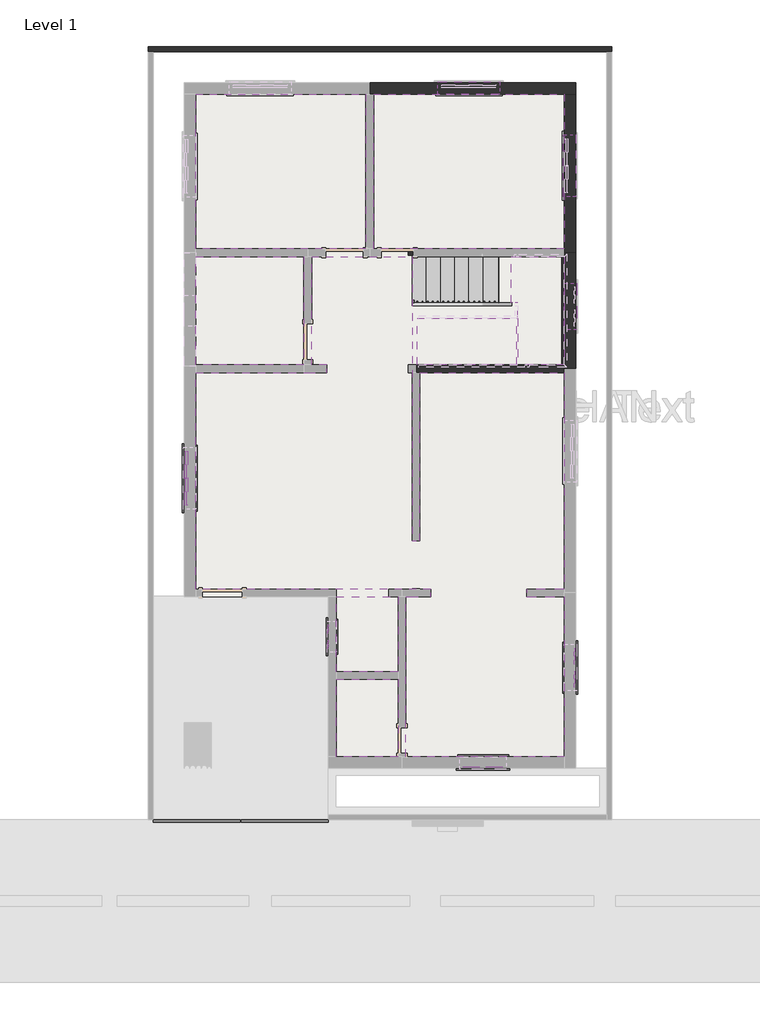
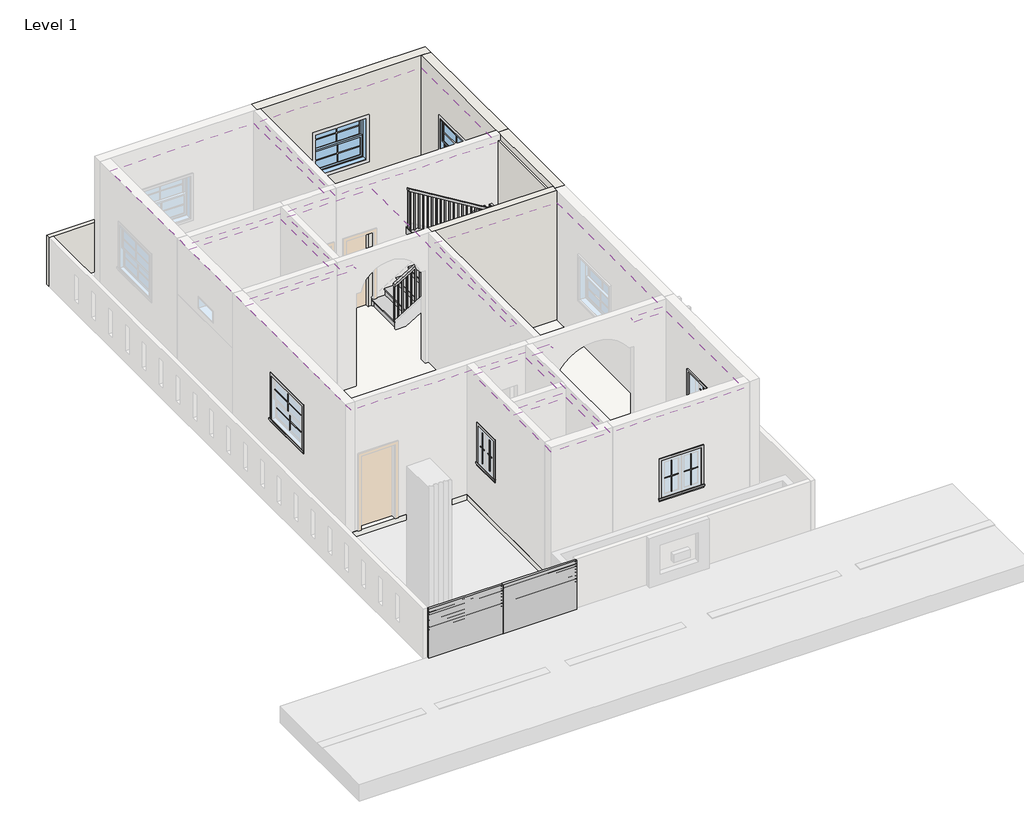
# One storey, part 2 of 3: 16 proxies, 8 walls, 6 coverings, 3 windows, 2 slabs, 2 stair flights, 1 furniture element, 1 railing.
"""IFC4 building model written with IfcOpenShell, lengths in millimetres."""

from ifc_helpers import new_model, si_unit, frame, origin, origin_with_axes, place, context, project, spatial, polyline, outline, extrude, faceted_brep, transform, mapped, element, save
from components import muntin_pattern_2x2_muntin_pattern_2x2_8b3f23e7, muntin_pattern_2x2_muntin_pattern_2x2_d1c6e638, muntin_pattern_2x2_muntin_pattern_2x2_37b95fb2, muntin_pattern_2x2_muntin_pattern_2x2_53152e2c, muntin_pattern_2x2_muntin_pattern_2x2_e8f3e573, trim_window_exterior_flat_with_sill_f44f30ad, trim_window_exterior_flat_with_sill_84e24481, trim_window_exterior_flat_with_sill_a665a915, trim_window_interior_flat_picture_frame_1dce1945, trim_window_interior_flat_picture_frame_28d4e5dc, trim_window_interior_flat_picture_frame_d485c387, casework_1_casework_1_032930e3, non_monolithic_landing_135adda5, stair_flight_5027378a, stair_flight_5d59741f, window_casement_double_3_90de19e9, window_double_hung_4_aab3aae7

model = new_model("IFC4")

# Units and contexts
model_context = context("Model", 3, world=origin())
ifc_project = project(units=[si_unit("LENGTHUNIT", "METRE", prefix="MILLI")], contexts=[model_context])

# Site, building, storey
site = spatial("IfcSite", under=ifc_project)
building = spatial("IfcBuilding", under=site)
storey = spatial("IfcBuildingStorey", under=building, Name="Level 1", Elevation=0.0)

# Proxies
placement = place(None, origin())
muntin_pattern_2x2_muntin_pattern_2x2_shape = muntin_pattern_2x2_muntin_pattern_2x2_8b3f23e7(model_context)
element("IfcBuildingElementProxy", 1, Name="Muntin Pattern_2x2 : Muntin Pattern_2x2", ObjectType="Muntin Pattern_2x2 : Muntin Pattern_2x2", at=placement, inside=storey, context=model_context, shape_type="MappedRepresentation", body=[
    mapped(muntin_pattern_2x2_muntin_pattern_2x2_shape, transform((-5865.439062, -1114.6142637, 1774.825), x_axis=(0.0, 1.0, 0.0), y_axis=(-1.0, 0.0, 0.0), z_axis=(0.0, 0.0, 1.0))),
])
element("IfcBuildingElementProxy", 2, Name="Muntin Pattern_2x2 : Muntin Pattern_2x2", ObjectType="Muntin Pattern_2x2 : Muntin Pattern_2x2", at=placement, inside=storey, context=model_context, shape_type="MappedRepresentation", body=[
    mapped(muntin_pattern_2x2_muntin_pattern_2x2_shape, transform((-5820.989062, -1114.6142637, 1295.4), x_axis=(0.0, 1.0, 0.0), y_axis=(-1.0, 0.0, 0.0), z_axis=(0.0, 0.0, 1.0))),
])
muntin_pattern_2x2_muntin_pattern_2x2_2_shape = muntin_pattern_2x2_muntin_pattern_2x2_d1c6e638(model_context)
element("IfcBuildingElementProxy", 3, Name="Muntin Pattern_2x2 : Muntin Pattern_2x2", ObjectType="Muntin Pattern_2x2 : Muntin Pattern_2x2", at=placement, inside=storey, context=model_context, shape_type="MappedRepresentation", body=[
    mapped(muntin_pattern_2x2_muntin_pattern_2x2_2_shape, transform((1811.710938, -4621.4017637, 1289.05), x_axis=(0.0, -1.0, 0.0), y_axis=(1.0, 0.0, 0.0), z_axis=(0.0, 0.0, 1.0))),
])
element("IfcBuildingElementProxy", 4, Name="Muntin Pattern_2x2 : Muntin Pattern_2x2", ObjectType="Muntin Pattern_2x2 : Muntin Pattern_2x2", at=placement, inside=storey, context=model_context, shape_type="MappedRepresentation", body=[
    mapped(muntin_pattern_2x2_muntin_pattern_2x2_2_shape, transform((219.448438, -6820.0892637, 1289.05), x_axis=(-1.0, 0.0, 0.0), y_axis=(0.0, -1.0, 0.0), z_axis=(0.0, 0.0, 1.0))),
])
muntin_pattern_2x2_muntin_pattern_2x2_3_shape = muntin_pattern_2x2_muntin_pattern_2x2_37b95fb2(model_context)
element("IfcBuildingElementProxy", 5, Name="Muntin Pattern_2x2 : Muntin Pattern_2x2", ObjectType="Muntin Pattern_2x2 : Muntin Pattern_2x2", at=placement, inside=storey, context=model_context, shape_type="MappedRepresentation", body=[
    mapped(muntin_pattern_2x2_muntin_pattern_2x2_3_shape, transform((1811.710938, -5075.4267637, 1289.05), x_axis=(0.0, 1.0, 0.0), y_axis=(-1.0, 0.0, 0.0), z_axis=(0.0, 0.0, 1.0))),
])
element("IfcBuildingElementProxy", 6, Name="Muntin Pattern_2x2 : Muntin Pattern_2x2", ObjectType="Muntin Pattern_2x2 : Muntin Pattern_2x2", at=placement, inside=storey, context=model_context, shape_type="MappedRepresentation", body=[
    mapped(muntin_pattern_2x2_muntin_pattern_2x2_3_shape, transform((-234.576562, -6820.0892637, 1289.05), x_axis=(1.0, 0.0, 0.0), y_axis=(0.0, 1.0, 0.0), z_axis=(0.0, 0.0, 1.0))),
])
muntin_pattern_2x2_muntin_pattern_2x2_4_shape = muntin_pattern_2x2_muntin_pattern_2x2_53152e2c(model_context)
element("IfcBuildingElementProxy", 7, Name="Muntin Pattern_2x2 : Muntin Pattern_2x2", ObjectType="Muntin Pattern_2x2 : Muntin Pattern_2x2", at=placement, inside=storey, context=model_context, shape_type="MappedRepresentation", body=[
    mapped(muntin_pattern_2x2_muntin_pattern_2x2_4_shape, transform((-3046.039062, -4389.6267637, 1289.05), x_axis=(0.0, 1.0, 0.0), y_axis=(-1.0, 0.0, 0.0), z_axis=(0.0, 0.0, 1.0))),
])
muntin_pattern_2x2_muntin_pattern_2x2_5_shape = muntin_pattern_2x2_muntin_pattern_2x2_e8f3e573(model_context)
element("IfcBuildingElementProxy", 8, Name="Muntin Pattern_2x2 : Muntin Pattern_2x2", ObjectType="Muntin Pattern_2x2 : Muntin Pattern_2x2", at=placement, inside=storey, context=model_context, shape_type="MappedRepresentation", body=[
    mapped(muntin_pattern_2x2_muntin_pattern_2x2_5_shape, transform((-3046.039062, -4088.0017637, 1289.05), x_axis=(0.0, -1.0, 0.0), y_axis=(1.0, 0.0, 0.0), z_axis=(0.0, 0.0, 1.0))),
])
trim_window_exterior_flat_with_sill_shape = trim_window_exterior_flat_with_sill_f44f30ad(model_context)
element("IfcBuildingElementProxy", 9, Name="Trim-Window-Exterior-Flat : with Sill", ObjectType="Trim-Window-Exterior-Flat : with Sill", at=placement, inside=storey, context=model_context, shape_type="MappedRepresentation", body=[
    mapped(trim_window_exterior_flat_with_sill_shape, transform((-5900.364062, -1114.6142637, 2286.0), x_axis=(0.0, -1.0, 0.0), y_axis=(0.0, 0.0, 1.0), z_axis=(-1.0, 0.0, 0.0))),
])
trim_window_exterior_flat_with_sill_2_shape = trim_window_exterior_flat_with_sill_84e24481(model_context)
element("IfcBuildingElementProxy", 10, Name="Trim-Window-Exterior-Flat : with Sill", ObjectType="Trim-Window-Exterior-Flat : with Sill", at=placement, inside=storey, context=model_context, shape_type="MappedRepresentation", body=[
    mapped(trim_window_exterior_flat_with_sill_2_shape, transform((1821.235938, -4848.4142637, 2133.6), x_axis=(0.0, 1.0, 0.0), y_axis=(0.0, 0.0, 1.0), z_axis=(1.0, 0.0, 0.0))),
])
element("IfcBuildingElementProxy", 11, Name="Trim-Window-Exterior-Flat : with Sill", ObjectType="Trim-Window-Exterior-Flat : with Sill", at=placement, inside=storey, context=model_context, shape_type="MappedRepresentation", body=[
    mapped(trim_window_exterior_flat_with_sill_2_shape, transform((-7.564062, -6829.6142637, 2133.6), x_axis=(1.0, 0.0, 0.0), y_axis=(0.0, 0.0, 1.0), z_axis=(0.0, -1.0, 0.0))),
])
trim_window_exterior_flat_with_sill_3_shape = trim_window_exterior_flat_with_sill_a665a915(model_context)
element("IfcBuildingElementProxy", 12, Name="Trim-Window-Exterior-Flat : with Sill", ObjectType="Trim-Window-Exterior-Flat : with Sill", at=placement, inside=storey, context=model_context, shape_type="MappedRepresentation", body=[
    mapped(trim_window_exterior_flat_with_sill_3_shape, transform((-3055.564062, -4238.8142637, 2133.6), x_axis=(0.0, -1.0, 0.0), y_axis=(0.0, 0.0, 1.0), z_axis=(-1.0, 0.0, 0.0))),
])
trim_window_interior_flat_picture_frame_shape = trim_window_interior_flat_picture_frame_1dce1945(model_context)
element("IfcBuildingElementProxy", 13, Name="Trim-Window-Interior-Flat : Picture Frame", ObjectType="Trim-Window-Interior-Flat : Picture Frame", at=placement, inside=storey, context=model_context, shape_type="MappedRepresentation", body=[
    mapped(trim_window_interior_flat_picture_frame_shape, transform((-5671.764062, -1114.6142637, 2286.0), x_axis=(0.0, 1.0, 0.0), y_axis=(0.0, 0.0, 1.0), z_axis=(1.0, 0.0, 0.0))),
])
trim_window_interior_flat_picture_frame_2_shape = trim_window_interior_flat_picture_frame_28d4e5dc(model_context)
element("IfcBuildingElementProxy", 14, Name="Trim-Window-Interior-Flat : Picture Frame", ObjectType="Trim-Window-Interior-Flat : Picture Frame", at=placement, inside=storey, context=model_context, shape_type="MappedRepresentation", body=[
    mapped(trim_window_interior_flat_picture_frame_2_shape, transform((1592.635938, -4848.4142637, 2133.6), x_axis=(0.0, -1.0, 0.0), y_axis=(0.0, 0.0, 1.0), z_axis=(-1.0, 0.0, 0.0))),
])
element("IfcBuildingElementProxy", 15, Name="Trim-Window-Interior-Flat : Picture Frame", ObjectType="Trim-Window-Interior-Flat : Picture Frame", at=placement, inside=storey, context=model_context, shape_type="MappedRepresentation", body=[
    mapped(trim_window_interior_flat_picture_frame_2_shape, transform((-7.564062, -6601.0142637, 2133.6), x_axis=(-1.0, 0.0, 0.0), y_axis=(0.0, 0.0, 1.0), z_axis=(0.0, 1.0, 0.0))),
])
trim_window_interior_flat_picture_frame_3_shape = trim_window_interior_flat_picture_frame_d485c387(model_context)
element("IfcBuildingElementProxy", 16, Name="Trim-Window-Interior-Flat : Picture Frame", ObjectType="Trim-Window-Interior-Flat : Picture Frame", at=placement, inside=storey, context=model_context, shape_type="MappedRepresentation", body=[
    mapped(trim_window_interior_flat_picture_frame_3_shape, transform((-2903.164062, -4238.8142637, 2133.6), x_axis=(0.0, 1.0, 0.0), y_axis=(0.0, 0.0, 1.0), z_axis=(1.0, 0.0, 0.0))),
])

# Coverings
element("IfcCovering", 17, ObjectType="2' x 4' ACT System", at=placement, inside=storey, context=model_context, shape_type="SweptSolid", body=[
    extrude(outline(polyline([(-5671.764062, 3406.5857363), (-5671.764062, 6454.5857363), (-2318.964062, 6454.5857363), (-2318.964062, 3406.5857363), (-3461.964062, 3406.5857363), (-5671.764062, 3406.5857363)])), frame((0.0, 0.0, 3048.0), z_axis=(0.0, 0.0, 1.0), x_axis=(1.0, 0.0, 0.0)), (0.0, 0.0, 1.0), 57.15),
])
element("IfcCovering", 18, ObjectType="2' x 4' ACT System", at=placement, inside=storey, context=model_context, shape_type="SweptSolid", body=[
    extrude(outline(polyline([(1592.635938, 6454.5857363), (1592.635938, 3406.5857363), (-2166.564062, 3406.5857363), (-2166.564062, 6454.5857363), (1592.635938, 6454.5857363)])), frame((0.0, 0.0, 3048.0), z_axis=(0.0, 0.0, 1.0), x_axis=(1.0, 0.0, 0.0)), (0.0, 0.0, 1.0), 57.15),
])
element("IfcCovering", 19, ObjectType="2' x 4' ACT System", at=placement, inside=storey, context=model_context, shape_type="SweptSolid", body=[
    extrude(outline(polyline([(-5671.764062, 1120.5857363), (-5671.764062, 3254.1857363), (-3538.164062, 3254.1857363), (-3538.164062, 1120.5857363), (-5671.764062, 1120.5857363)])), frame((0.0, 0.0, 3048.0), z_axis=(0.0, 0.0, 1.0), x_axis=(1.0, 0.0, 0.0)), (0.0, 0.0, 1.0), 57.15),
])
element("IfcCovering", 20, ObjectType="2' x 4' ACT System", at=placement, inside=storey, context=model_context, shape_type="SweptSolid", body=[
    extrude(outline(polyline([(1592.635938, -3451.4142637), (1592.635938, -6601.0142637), (-1531.564062, -6601.0142637), (-1531.564062, -3451.4142637), (-1042.9877715, -3451.4142637), (-1042.9877715, -3299.0142637), (-1607.764062, -3299.0142637), (-5671.764062, -3299.0142637), (-5671.764062, 968.1857363), (-3538.164062, 968.1857363), (-3088.5741654, 968.1857363), (-3088.5741654, 1120.5857363), (-3385.764062, 1120.5857363), (-3385.764062, 3254.1857363), (-2242.764062, 3254.1857363), (-1404.564062, 3254.1857363), (-1404.564062, -2346.4297845), (-1252.164062, -2346.4297845), (-1252.164062, 968.1857363), (1592.635938, 968.1857363), (1592.635938, -3299.0142637), (852.655246, -3299.0142637), (852.655246, -3451.4142637), (1592.635938, -3451.4142637)])), frame((0.0, 0.0, 3048.0), z_axis=(0.0, 0.0, 1.0), x_axis=(1.0, 0.0, 0.0)), (0.0, 0.0, 1.0), 57.15),
])
element("IfcCovering", 21, ObjectType="2' x 4' ACT System", at=placement, inside=storey, context=model_context, shape_type="SweptSolid", body=[
    extrude(outline(polyline([(-2903.164062, -4924.6142637), (-2903.164062, -3451.4142637), (-1683.964062, -3451.4142637), (-1683.964062, -4924.6142637), (-2903.164062, -4924.6142637)])), frame((0.0, 0.0, 3048.0), z_axis=(0.0, 0.0, 1.0), x_axis=(1.0, 0.0, 0.0)), (0.0, 0.0, 1.0), 57.15),
])
element("IfcCovering", 22, ObjectType="2' x 4' ACT System", at=placement, inside=storey, context=model_context, shape_type="SweptSolid", body=[
    extrude(outline(polyline([(-2903.164062, -6601.0142637), (-2903.164062, -5077.0142637), (-1683.964062, -5077.0142637), (-1683.964062, -6601.0142637), (-2903.164062, -6601.0142637)])), frame((0.0, 0.0, 3048.0), z_axis=(0.0, 0.0, 1.0), x_axis=(1.0, 0.0, 0.0)), (0.0, 0.0, 1.0), 57.15),
])

# Furniture
casework_1_casework_1_shape = casework_1_casework_1_032930e3(model_context)
element("IfcFurniture", 23, ObjectType="Casework 1 : Casework 1", at=placement, inside=storey, context=model_context, shape_type="MappedRepresentation", body=[
    mapped(casework_1_casework_1_shape, transform((0.0, 0.0, 0.0), x_axis=(1.0, 0.0, 0.0), y_axis=(0.0, 1.0, 0.0), z_axis=(0.0, 0.0, 1.0))),
])

# Railing
element("IfcRailing", 24, ObjectType="Handrail - Rectangular", at=placement, inside=storey, context=model_context, shape_type="SolidModel", body=[
    faceted_brep([(-1404.564062, 2390.5857363, 1236.1333333), (-1404.564062, 2390.5857363, 1176.7318731), (-1404.564062, 2339.7857363, 1176.7318731), (-1404.564062, 2339.7857363, 1236.1333333), (551.235938, 2390.5857363, 2421.4666667), (565.4283474, 2390.5857363, 2370.6666667), (565.4283474, 2339.7857363, 2370.6666667), (551.235938, 2339.7857363, 2421.4666667), (729.035938, 2390.5857363, 2421.4666667), (729.035938, 2390.5857363, 2370.6666667), (678.235938, 2339.7857363, 2370.6666667), (678.235938, 2339.7857363, 2421.4666667), (729.035938, 2111.1857363, 2421.4666667), (729.035938, 2060.3857363, 2370.6666667), (678.235938, 2060.3857363, 2370.6666667), (678.235938, 2111.1857363, 2421.4666667), (729.035938, 2111.1857363, 2636.9818182), (729.035938, 2060.3857363, 2586.1818182), (678.235938, 2060.3857363, 2586.1818182), (678.235938, 2111.1857363, 2636.9818182), (729.035938, 1984.1857363, 2636.9818182), (729.035938, 1984.1857363, 2586.1818182), (678.235938, 2034.9857363, 2586.1818182), (678.235938, 2034.9857363, 2636.9818182), (602.035938, 1984.1857363, 2636.9818182), (587.8435285, 1984.1857363, 2586.1818182), (587.8435285, 2034.9857363, 2586.1818182), (602.035938, 2034.9857363, 2636.9818182), (-1277.564062, 1984.1857363, 3776.1333333), (-1277.564062, 2034.9857363, 3776.1333333), (-1277.564062, 2034.9857363, 3716.7318731), (-1277.564062, 1984.1857363, 3716.7318731)], [[[0, 1, 2, 3]], [[1, 0, 4, 5]], [[2, 1, 5, 6]], [[3, 2, 6, 7]], [[0, 3, 7, 4]], [[5, 4, 8, 9]], [[6, 5, 9, 10]], [[7, 6, 10, 11]], [[4, 7, 11, 8]], [[9, 8, 12, 13]], [[10, 9, 13, 14]], [[11, 10, 14, 15]], [[8, 11, 15, 12]], [[13, 12, 16, 17]], [[14, 13, 17, 18]], [[15, 14, 18, 19]], [[12, 15, 19, 16]], [[17, 16, 20, 21]], [[18, 17, 21, 22]], [[19, 18, 22, 23]], [[16, 19, 23, 20]], [[21, 20, 24, 25]], [[22, 21, 25, 26]], [[23, 22, 26, 27]], [[20, 23, 27, 24]], [[28, 29, 30, 31]], [[25, 24, 28, 31]], [[26, 25, 31, 30]], [[27, 26, 30, 29]], [[24, 27, 29, 28]]]),
    extrude(outline(polyline([(3680.171267, -1217.239062), (3691.7167216, -1236.289062), (2692.4, -1236.289062), (2692.4, -1217.239062), (3680.171267, -1217.239062)])), frame((0.0, 2000.0607363, 0.0), z_axis=(0.0, 1.0, 0.0), x_axis=(0.0, 0.0, 1.0)), (0.0, 0.0, 1.0), 19.05),
    extrude(outline(polyline([(3618.5955094, -1115.639062), (3630.140964, -1134.689062), (2692.4, -1134.689062), (2692.4, -1115.639062), (3618.5955094, -1115.639062)])), frame((0.0, 2000.0607363, 0.0), z_axis=(0.0, 1.0, 0.0), x_axis=(0.0, 0.0, 1.0)), (0.0, 0.0, 1.0), 19.05),
    extrude(outline(polyline([(3557.0197519, -1014.039062), (3568.5652064, -1033.089062), (2692.4, -1033.089062), (2692.4, -1014.039062), (3557.0197519, -1014.039062)])), frame((0.0, 2000.0607363, 0.0), z_axis=(0.0, 1.0, 0.0), x_axis=(0.0, 0.0, 1.0)), (0.0, 0.0, 1.0), 19.05),
    extrude(outline(polyline([(3495.4439943, -912.439062), (3506.9894488, -931.489062), (2523.0666667, -931.489062), (2523.0666667, -912.439062), (3495.4439943, -912.439062)])), frame((0.0, 2000.0607363, 0.0), z_axis=(0.0, 1.0, 0.0), x_axis=(0.0, 0.0, 1.0)), (0.0, 0.0, 1.0), 19.05),
    extrude(outline(polyline([(3433.8682367, -810.839062), (3445.4136913, -829.889062), (2523.0666667, -829.889062), (2523.0666667, -810.839062), (3433.8682367, -810.839062)])), frame((0.0, 2000.0607363, 0.0), z_axis=(0.0, 1.0, 0.0), x_axis=(0.0, 0.0, 1.0)), (0.0, 0.0, 1.0), 19.05),
    extrude(outline(polyline([(3372.2924791, -709.239062), (3383.8379337, -728.289062), (2523.0666667, -728.289062), (2523.0666667, -709.239062), (3372.2924791, -709.239062)])), frame((0.0, 2000.0607363, 0.0), z_axis=(0.0, 1.0, 0.0), x_axis=(0.0, 0.0, 1.0)), (0.0, 0.0, 1.0), 19.05),
    extrude(outline(polyline([(3310.7167216, -607.639062), (3322.2621761, -626.689062), (2353.7333333, -626.689062), (2353.7333333, -607.639062), (3310.7167216, -607.639062)])), frame((0.0, 2000.0607363, 0.0), z_axis=(0.0, 1.0, 0.0), x_axis=(0.0, 0.0, 1.0)), (0.0, 0.0, 1.0), 19.05),
    extrude(outline(polyline([(3249.140964, -506.039062), (3260.6864185, -525.089062), (2353.7333333, -525.089062), (2353.7333333, -506.039062), (3249.140964, -506.039062)])), frame((0.0, 2000.0607363, 0.0), z_axis=(0.0, 1.0, 0.0), x_axis=(0.0, 0.0, 1.0)), (0.0, 0.0, 1.0), 19.05),
    extrude(outline(polyline([(3187.5652064, -404.439062), (3199.110661, -423.489062), (2184.4, -423.489062), (2184.4, -404.439062), (3187.5652064, -404.439062)])), frame((0.0, 2000.0607363, 0.0), z_axis=(0.0, 1.0, 0.0), x_axis=(0.0, 0.0, 1.0)), (0.0, 0.0, 1.0), 19.05),
    extrude(outline(polyline([(3125.9894488, -302.839062), (3137.5349034, -321.889062), (2184.4, -321.889062), (2184.4, -302.839062), (3125.9894488, -302.839062)])), frame((0.0, 2000.0607363, 0.0), z_axis=(0.0, 1.0, 0.0), x_axis=(0.0, 0.0, 1.0)), (0.0, 0.0, 1.0), 19.05),
    extrude(outline(polyline([(3064.4136913, -201.239062), (3075.9591458, -220.289062), (2184.4, -220.289062), (2184.4, -201.239062), (3064.4136913, -201.239062)])), frame((0.0, 2000.0607363, 0.0), z_axis=(0.0, 1.0, 0.0), x_axis=(0.0, 0.0, 1.0)), (0.0, 0.0, 1.0), 19.05),
    extrude(outline(polyline([(3002.8379337, -99.639062), (3014.3833882, -118.689062), (2015.0666667, -118.689062), (2015.0666667, -99.639062), (3002.8379337, -99.639062)])), frame((0.0, 2000.0607363, 0.0), z_axis=(0.0, 1.0, 0.0), x_axis=(0.0, 0.0, 1.0)), (0.0, 0.0, 1.0), 19.05),
    extrude(outline(polyline([(2941.2621761, 1.960938), (2952.8076307, -17.089062), (2015.0666667, -17.089062), (2015.0666667, 1.960938), (2941.2621761, 1.960938)])), frame((0.0, 2000.0607363, 0.0), z_axis=(0.0, 1.0, 0.0), x_axis=(0.0, 0.0, 1.0)), (0.0, 0.0, 1.0), 19.05),
    extrude(outline(polyline([(2879.6864185, 103.560938), (2891.2318731, 84.510938), (2015.0666667, 84.510938), (2015.0666667, 103.560938), (2879.6864185, 103.560938)])), frame((0.0, 2000.0607363, 0.0), z_axis=(0.0, 1.0, 0.0), x_axis=(0.0, 0.0, 1.0)), (0.0, 0.0, 1.0), 19.05),
    extrude(outline(polyline([(2818.110661, 205.160938), (2829.6561155, 186.110938), (1845.7333333, 186.110938), (1845.7333333, 205.160938), (2818.110661, 205.160938)])), frame((0.0, 2000.0607363, 0.0), z_axis=(0.0, 1.0, 0.0), x_axis=(0.0, 0.0, 1.0)), (0.0, 0.0, 1.0), 19.05),
    extrude(outline(polyline([(2756.5349034, 306.760938), (2768.0803579, 287.710938), (1845.7333333, 287.710938), (1845.7333333, 306.760938), (2756.5349034, 306.760938)])), frame((0.0, 2000.0607363, 0.0), z_axis=(0.0, 1.0, 0.0), x_axis=(0.0, 0.0, 1.0)), (0.0, 0.0, 1.0), 19.05),
    extrude(outline(polyline([(2694.9591458, 408.360938), (2706.5046004, 389.310938), (1845.7333333, 389.310938), (1845.7333333, 408.360938), (2694.9591458, 408.360938)])), frame((0.0, 2000.0607363, 0.0), z_axis=(0.0, 1.0, 0.0), x_axis=(0.0, 0.0, 1.0)), (0.0, 0.0, 1.0), 19.05),
    extrude(outline(polyline([(2633.3833882, 509.960938), (2644.9288428, 490.910938), (1676.4, 490.910938), (1676.4, 509.960938), (2633.3833882, 509.960938)])), frame((0.0, 2000.0607363, 0.0), z_axis=(0.0, 1.0, 0.0), x_axis=(0.0, 0.0, 1.0)), (0.0, 0.0, 1.0), 19.05),
    extrude(outline(polyline([(2571.8076307, 611.560938), (2583.3530852, 592.510938), (1676.4, 592.510938), (1676.4, 611.560938), (2571.8076307, 611.560938)])), frame((0.0, 2000.0607363, 0.0), z_axis=(0.0, 1.0, 0.0), x_axis=(0.0, 0.0, 1.0)), (0.0, 0.0, 1.0), 19.05),
    extrude(outline(polyline([(694.110938, 2069.9107363), (713.160938, 2069.9107363), (713.160938, 2050.8607363), (694.110938, 2050.8607363), (694.110938, 2069.9107363)])), frame((0.0, 0.0, 1507.0666667), z_axis=(0.0, 0.0, 1.0), x_axis=(1.0, 0.0, 0.0)), (0.0, 0.0, 1.0), 1079.1151515),
    extrude(outline(polyline([(694.110938, 2171.5107363), (713.160938, 2171.5107363), (713.160938, 2152.4607363), (694.110938, 2152.4607363), (694.110938, 2171.5107363)])), frame((0.0, 0.0, 1507.0666667), z_axis=(0.0, 0.0, 1.0), x_axis=(1.0, 0.0, 0.0)), (0.0, 0.0, 1.0), 863.6),
    extrude(outline(polyline([(694.110938, 2273.1107363), (713.160938, 2273.1107363), (713.160938, 2254.0607363), (694.110938, 2254.0607363), (694.110938, 2273.1107363)])), frame((0.0, 0.0, 1507.0666667), z_axis=(0.0, 0.0, 1.0), x_axis=(1.0, 0.0, 0.0)), (0.0, 0.0, 1.0), 863.6),
    extrude(outline(polyline([(643.310938, 2355.6607363), (643.310938, 2374.7107363), (662.360938, 2374.7107363), (662.360938, 2355.6607363), (643.310938, 2355.6607363)])), frame((0.0, 0.0, 1507.0666667), z_axis=(0.0, 0.0, 1.0), x_axis=(1.0, 0.0, 0.0)), (0.0, 0.0, 1.0), 863.6),
    extrude(outline(polyline([(2352.4439943, 535.360938), (2340.8985397, 516.310938), (1337.7333333, 516.310938), (1337.7333333, 535.360938), (2352.4439943, 535.360938)])), frame((0.0, 2355.6607363, 0.0), z_axis=(0.0, 1.0, 0.0), x_axis=(0.0, 0.0, 1.0)), (0.0, 0.0, 1.0), 19.05),
    extrude(outline(polyline([(2290.8682367, 433.760938), (2279.3227822, 414.710938), (1337.7333333, 414.710938), (1337.7333333, 433.760938), (2290.8682367, 433.760938)])), frame((0.0, 2355.6607363, 0.0), z_axis=(0.0, 1.0, 0.0), x_axis=(0.0, 0.0, 1.0)), (0.0, 0.0, 1.0), 19.05),
    extrude(outline(polyline([(2229.2924791, 332.160938), (2217.7470246, 313.110938), (1337.7333333, 313.110938), (1337.7333333, 332.160938), (2229.2924791, 332.160938)])), frame((0.0, 2355.6607363, 0.0), z_axis=(0.0, 1.0, 0.0), x_axis=(0.0, 0.0, 1.0)), (0.0, 0.0, 1.0), 19.05),
    extrude(outline(polyline([(2167.7167216, 230.560938), (2156.171267, 211.510938), (1168.4, 211.510938), (1168.4, 230.560938), (2167.7167216, 230.560938)])), frame((0.0, 2355.6607363, 0.0), z_axis=(0.0, 1.0, 0.0), x_axis=(0.0, 0.0, 1.0)), (0.0, 0.0, 1.0), 19.05),
    extrude(outline(polyline([(2106.140964, 128.960938), (2094.5955094, 109.910938), (1168.4, 109.910938), (1168.4, 128.960938), (2106.140964, 128.960938)])), frame((0.0, 2355.6607363, 0.0), z_axis=(0.0, 1.0, 0.0), x_axis=(0.0, 0.0, 1.0)), (0.0, 0.0, 1.0), 19.05),
    extrude(outline(polyline([(2044.5652064, 27.360938), (2033.0197519, 8.310938), (1168.4, 8.310938), (1168.4, 27.360938), (2044.5652064, 27.360938)])), frame((0.0, 2355.6607363, 0.0), z_axis=(0.0, 1.0, 0.0), x_axis=(0.0, 0.0, 1.0)), (0.0, 0.0, 1.0), 19.05),
    extrude(outline(polyline([(1982.9894488, -74.239062), (1971.4439943, -93.289062), (999.0666667, -93.289062), (999.0666667, -74.239062), (1982.9894488, -74.239062)])), frame((0.0, 2355.6607363, 0.0), z_axis=(0.0, 1.0, 0.0), x_axis=(0.0, 0.0, 1.0)), (0.0, 0.0, 1.0), 19.05),
    extrude(outline(polyline([(1921.4136913, -175.839062), (1909.8682367, -194.889062), (999.0666667, -194.889062), (999.0666667, -175.839062), (1921.4136913, -175.839062)])), frame((0.0, 2355.6607363, 0.0), z_axis=(0.0, 1.0, 0.0), x_axis=(0.0, 0.0, 1.0)), (0.0, 0.0, 1.0), 19.05),
    extrude(outline(polyline([(1859.8379337, -277.439062), (1848.2924791, -296.489062), (999.0666667, -296.489062), (999.0666667, -277.439062), (1859.8379337, -277.439062)])), frame((0.0, 2355.6607363, 0.0), z_axis=(0.0, 1.0, 0.0), x_axis=(0.0, 0.0, 1.0)), (0.0, 0.0, 1.0), 19.05),
    extrude(outline(polyline([(1798.2621761, -379.039062), (1786.7167216, -398.089062), (829.7333333, -398.089062), (829.7333333, -379.039062), (1798.2621761, -379.039062)])), frame((0.0, 2355.6607363, 0.0), z_axis=(0.0, 1.0, 0.0), x_axis=(0.0, 0.0, 1.0)), (0.0, 0.0, 1.0), 19.05),
    extrude(outline(polyline([(1736.6864185, -480.639062), (1725.140964, -499.689062), (829.7333333, -499.689062), (829.7333333, -480.639062), (1736.6864185, -480.639062)])), frame((0.0, 2355.6607363, 0.0), z_axis=(0.0, 1.0, 0.0), x_axis=(0.0, 0.0, 1.0)), (0.0, 0.0, 1.0), 19.05),
    extrude(outline(polyline([(1675.110661, -582.239062), (1663.5652064, -601.289062), (660.4, -601.289062), (660.4, -582.239062), (1675.110661, -582.239062)])), frame((0.0, 2355.6607363, 0.0), z_axis=(0.0, 1.0, 0.0), x_axis=(0.0, 0.0, 1.0)), (0.0, 0.0, 1.0), 19.05),
    extrude(outline(polyline([(1613.5349034, -683.839062), (1601.9894488, -702.889062), (660.4, -702.889062), (660.4, -683.839062), (1613.5349034, -683.839062)])), frame((0.0, 2355.6607363, 0.0), z_axis=(0.0, 1.0, 0.0), x_axis=(0.0, 0.0, 1.0)), (0.0, 0.0, 1.0), 19.05),
    extrude(outline(polyline([(1551.9591458, -785.439062), (1540.4136913, -804.489062), (660.4, -804.489062), (660.4, -785.439062), (1551.9591458, -785.439062)])), frame((0.0, 2355.6607363, 0.0), z_axis=(0.0, 1.0, 0.0), x_axis=(0.0, 0.0, 1.0)), (0.0, 0.0, 1.0), 19.05),
    extrude(outline(polyline([(1490.3833882, -887.039062), (1478.8379337, -906.089062), (491.0666667, -906.089062), (491.0666667, -887.039062), (1490.3833882, -887.039062)])), frame((0.0, 2355.6607363, 0.0), z_axis=(0.0, 1.0, 0.0), x_axis=(0.0, 0.0, 1.0)), (0.0, 0.0, 1.0), 19.05),
    extrude(outline(polyline([(1428.8076307, -988.639062), (1417.2621761, -1007.689062), (491.0666667, -1007.689062), (491.0666667, -988.639062), (1428.8076307, -988.639062)])), frame((0.0, 2355.6607363, 0.0), z_axis=(0.0, 1.0, 0.0), x_axis=(0.0, 0.0, 1.0)), (0.0, 0.0, 1.0), 19.05),
    extrude(outline(polyline([(1367.2318731, -1090.239062), (1355.6864185, -1109.289062), (491.0666667, -1109.289062), (491.0666667, -1090.239062), (1367.2318731, -1090.239062)])), frame((0.0, 2355.6607363, 0.0), z_axis=(0.0, 1.0, 0.0), x_axis=(0.0, 0.0, 1.0)), (0.0, 0.0, 1.0), 19.05),
    extrude(outline(polyline([(1305.6561155, -1191.839062), (1294.110661, -1210.889062), (321.7333333, -1210.889062), (321.7333333, -1191.839062), (1305.6561155, -1191.839062)])), frame((0.0, 2355.6607363, 0.0), z_axis=(0.0, 1.0, 0.0), x_axis=(0.0, 0.0, 1.0)), (0.0, 0.0, 1.0), 19.05),
    extrude(outline(polyline([(1244.0803579, -1293.439062), (1232.5349034, -1312.489062), (321.7333333, -1312.489062), (321.7333333, -1293.439062), (1244.0803579, -1293.439062)])), frame((0.0, 2355.6607363, 0.0), z_axis=(0.0, 1.0, 0.0), x_axis=(0.0, 0.0, 1.0)), (0.0, 0.0, 1.0), 19.05),
    extrude(outline(polyline([(694.110938, 2019.1107363), (713.160938, 2019.1107363), (713.160938, 2000.0607363), (694.110938, 2000.0607363), (694.110938, 2019.1107363)])), frame((0.0, 0.0, 1507.0666667), z_axis=(0.0, 0.0, 1.0), x_axis=(1.0, 0.0, 0.0)), (0.0, 0.0, 1.0), 1079.1151515),
    extrude(outline(polyline([(694.110938, 2355.6607363), (694.110938, 2374.7107363), (713.160938, 2374.7107363), (713.160938, 2355.6607363), (694.110938, 2355.6607363)])), frame((0.0, 0.0, 1507.0666667), z_axis=(0.0, 0.0, 1.0), x_axis=(1.0, 0.0, 0.0)), (0.0, 0.0, 1.0), 863.6),
    extrude(outline(polyline([(2367.8379337, 560.760938), (2356.2924791, 541.710938), (1507.0666667, 541.710938), (1507.0666667, 560.760938), (2367.8379337, 560.760938)])), frame((0.0, 2355.6607363, 0.0), z_axis=(0.0, 1.0, 0.0), x_axis=(0.0, 0.0, 1.0)), (0.0, 0.0, 1.0), 19.05),
    extrude(outline(polyline([(3705.1864185, -1258.514062), (3716.7318731, -1277.564062), (2692.4, -1277.564062), (2692.4, -1258.514062), (3705.1864185, -1258.514062)])), frame((0.0, 2000.0607363, 0.0), z_axis=(0.0, 1.0, 0.0), x_axis=(0.0, 0.0, 1.0)), (0.0, 0.0, 1.0), 19.05),
    extrude(outline(polyline([(1188.2773276, -1385.514062), (1176.7318731, -1404.564062), (321.7333333, -1404.564062), (321.7333333, -1385.514062), (1188.2773276, -1385.514062)])), frame((0.0, 2355.6607363, 0.0), z_axis=(0.0, 1.0, 0.0), x_axis=(0.0, 0.0, 1.0)), (0.0, 0.0, 1.0), 19.05),
])

# Slabs
element("IfcSlab", 25, ObjectType="Generic - 6\"", at=placement, inside=storey, context=model_context, shape_type="SweptSolid", body=[
    extrude(outline(polyline([(-5900.364062, -3451.4142637), (-5900.364062, 6683.1857363), (1821.235938, 6683.1857363), (1821.235938, -6829.6142637), (-3055.564062, -6829.6142637), (-3055.564062, -3451.4142637), (-5900.364062, -3451.4142637)])), origin_with_axes(), (0.0, 0.0, 1.0), 152.4),
])
non_monolithic_landing_shape = non_monolithic_landing_135adda5(model_context)
element("IfcSlab", 26, ObjectType="Non-Monolithic Landing", at=placement, inside=storey, context=model_context, shape_type="MappedRepresentation", body=[
    mapped(non_monolithic_landing_shape, transform((0.0, 0.0, 0.0), x_axis=(1.0, 0.0, 0.0), y_axis=(0.0, 1.0, 0.0), z_axis=(0.0, 0.0, 1.0))),
])

# Stair flights
stair_flight_shape = stair_flight_5027378a(model_context)
element("IfcStairFlight", 27, ObjectType="2\" Tread 1\" Nosing 1/4\" Riser", at=placement, inside=storey, context=model_context, shape_type="MappedRepresentation", body=[
    mapped(stair_flight_shape, transform((0.0, 0.0, 0.0), x_axis=(1.0, 0.0, 0.0), y_axis=(0.0, 1.0, 0.0), z_axis=(0.0, 0.0, 1.0))),
])
stair_flight_2_shape = stair_flight_5d59741f(model_context)
element("IfcStairFlight", 28, ObjectType="2\" Tread 1\" Nosing 1/4\" Riser", at=placement, inside=storey, context=model_context, shape_type="MappedRepresentation", body=[
    mapped(stair_flight_2_shape, transform((0.0, 0.0, 0.0), x_axis=(1.0, 0.0, 0.0), y_axis=(0.0, 1.0, 0.0), z_axis=(0.0, 0.0, 1.0))),
])

# Walls
element("IfcWall", 29, ObjectType="Generic - 4\"", at=placement, inside=storey, context=model_context, shape_type="Brep", body=[
    faceted_brep([(-6611.564062, 7292.7857363, 0.0), (-6509.964062, 7292.7857363, 0.0), (2430.835938, 7292.7857363, 0.0), (2532.435938, 7292.7857363, 0.0), (2532.435938, 7292.7857363, 1219.2), (2430.835938, 7292.7857363, 1219.2), (-6509.964062, 7292.7857363, 1219.2), (-6611.564062, 7292.7857363, 1219.2), (-6611.564062, 7394.3857363, 0.0), (-6611.564062, 7394.3857363, 1219.2), (2532.435938, 7394.3857363, 1219.2), (2532.435938, 7394.3857363, 0.0)], [[[0, 1, 2, 3, 4, 5, 6, 7]], [[8, 9, 10, 11]], [[3, 2, 1, 0, 8, 11]], [[7, 6, 5, 4, 10, 9]], [[4, 3, 11, 10]], [[0, 7, 9, 8]]]),
])
element("IfcWall", 30, ObjectType="Generic - 4\"", at=placement, inside=storey, context=model_context, shape_type="Brep", body=[
    faceted_brep([(1643.435938, 3381.1857363, 0.0), (-1480.764062, 3381.1857363, 0.0), (-1480.764062, 3381.1857363, 3200.4), (1592.635938, 3381.1857363, 3200.4), (1592.635938, 3381.1857363, 152.4), (1643.435938, 3381.1857363, 152.4), (1643.435938, 3279.5857363, 0.0), (1643.435938, 3279.5857363, 152.4), (1592.635938, 3279.5857363, 152.4), (1592.635938, 3279.5857363, 3200.4), (-1480.764062, 3279.5857363, 3200.4), (-1480.764062, 3279.5857363, 0.0), (1541.835938, 3279.5857363, 0.0), (1592.635938, 3330.3857363, 152.4)], [[[0, 1, 2, 3, 4, 5]], [[6, 7, 8, 9, 10, 11, 12]], [[1, 0, 6, 12, 11]], [[2, 1, 11, 10]], [[3, 2, 10, 9]], [[4, 13, 8, 7, 5]], [[0, 5, 7, 6]], [[4, 3, 9, 8, 13]]]),
])
element("IfcWall", 31, ObjectType="Generic - 4\"", at=placement, inside=storey, context=model_context, shape_type="Brep", body=[
    faceted_brep([(1643.435938, 993.5857363, 0.0), (1643.435938, 3279.5857363, 0.0), (1643.435938, 3279.5857363, 152.4), (1643.435938, 3254.1857363, 152.4), (1643.435938, 3254.1857363, 3200.4), (1643.435938, 1120.5857363, 3200.4), (1643.435938, 1120.5857363, 152.4), (1643.435938, 993.5857363, 152.4), (1541.835938, 993.5857363, 0.0), (1541.835938, 993.5857363, 152.4), (1541.835938, 1095.1857363, 152.4), (1541.835938, 1120.5857363, 152.4), (1541.835938, 1120.5857363, 3200.4), (1541.835938, 3254.1857363, 3200.4), (1541.835938, 3254.1857363, 152.4), (1541.835938, 3279.5857363, 152.4), (1541.835938, 3279.5857363, 0.0), (1541.835938, 1095.1857363, 0.0), (1592.635938, 3254.1857363, 152.4), (1592.635938, 3279.5857363, 152.4), (1592.635938, 1120.5857363, 152.4), (1592.635938, 993.5857363, 152.4)], [[[0, 1, 2, 3, 4, 5, 6, 7]], [[8, 9, 10, 11, 12, 13, 14, 15, 16, 17]], [[1, 0, 8, 17, 16]], [[5, 4, 13, 12]], [[14, 18, 3, 2, 19, 15]], [[2, 1, 16, 15, 19]], [[4, 3, 18, 14, 13]], [[6, 20, 11, 10, 9, 21, 7]], [[0, 7, 21, 9, 8]], [[6, 5, 12, 11, 20]]]),
])
element("IfcWall", 32, ObjectType="Generic - 4\"", at=placement, inside=storey, context=model_context, shape_type="Brep", body=[
    faceted_brep([(-1480.764062, 993.5857363, 3200.4), (-1480.764062, 993.5857363, 0.0), (1541.835938, 993.5857363, 0.0), (1541.835938, 993.5857363, 152.4), (1592.635938, 993.5857363, 152.4), (1592.635938, 993.5857363, 3200.4), (-1480.764062, 1095.1857363, 0.0), (-1480.764062, 1095.1857363, 3200.4), (1592.635938, 1095.1857363, 3200.4), (1592.635938, 1095.1857363, 152.4), (1541.835938, 1095.1857363, 152.4), (1541.835938, 1095.1857363, 0.0), (1592.635938, 1044.3857363, 152.4)], [[[0, 1, 2, 3, 4, 5]], [[6, 7, 8, 9, 10, 11]], [[2, 1, 6, 11]], [[0, 5, 8, 7]], [[0, 7, 6, 1]], [[9, 12, 4, 3, 10]], [[3, 2, 11, 10]], [[5, 4, 12, 9, 8]]]),
])
element("IfcWall", 33, ObjectType="Generic - 6\"", at=placement, inside=storey, context=model_context, shape_type="Brep", body=[
    faceted_brep([(1592.635938, 968.1857363, 152.4), (1592.635938, 968.1857363, 3352.8), (-1252.164062, 968.1857363, 3352.8), (-1328.364062, 968.1857363, 3352.8), (-1328.364062, 968.1857363, 152.4), (-1252.164062, 968.1857363, 152.4), (1592.635938, 1120.5857363, 3352.8), (1592.635938, 1120.5857363, 152.4), (1541.835938, 1120.5857363, 152.4), (-1328.364062, 1120.5857363, 152.4), (-1328.364062, 1120.5857363, 3352.8), (1592.635938, 1044.3857363, 3352.8), (1592.635938, 1044.3857363, 152.4)], [[[0, 1, 2, 3, 4, 5]], [[6, 7, 8, 9, 10]], [[3, 2, 1, 11, 6, 10]], [[0, 5, 4, 9, 8, 7, 12]], [[3, 10, 9, 4]], [[0, 12, 7, 6, 11, 1]]]),
])
element("IfcWall", 34, ObjectType="Generic - 9\"", at=placement, inside=storey, context=model_context, shape_type="Brep", body=[
    faceted_brep([(1592.635938, 6454.5857363, 152.4), (1592.635938, 3406.5857363, 152.4), (1592.635938, 3381.1857363, 152.4), (1592.635938, 3330.3857363, 152.4), (1592.635938, 3330.3857363, 3352.8), (1592.635938, 3406.5857363, 3352.8), (1592.635938, 6454.5857363, 3352.8), (1592.635938, 5654.4857363, 2286.0), (1592.635938, 4435.2857363, 2286.0), (1592.635938, 4435.2857363, 1219.2), (1592.635938, 5654.4857363, 1219.2), (1821.235938, 6454.5857363, 152.4), (1821.235938, 6454.5857363, 3352.8), (1821.235938, 3330.3857363, 3352.8), (1821.235938, 3330.3857363, 152.4), (1821.235938, 5654.4857363, 2286.0), (1821.235938, 5654.4857363, 1219.2), (1821.235938, 4435.2857363, 1219.2), (1821.235938, 4435.2857363, 2286.0)], [[[0, 1, 2, 3, 4, 5, 6], [7, 8, 9, 10]], [[11, 12, 13, 14], [15, 16, 17, 18]], [[3, 2, 1, 0, 11, 14]], [[6, 5, 4, 13, 12]], [[0, 6, 12, 11]], [[16, 15, 7, 10]], [[17, 16, 10, 9]], [[18, 17, 9, 8]], [[15, 18, 8, 7]], [[3, 14, 13, 4]]]),
])
element("IfcWall", 35, ObjectType="Generic - 9\"", at=placement, inside=storey, context=model_context, shape_type="Brep", body=[
    faceted_brep([(-2242.764062, 6454.5857363, 152.4), (-2166.564062, 6454.5857363, 152.4), (1592.635938, 6454.5857363, 152.4), (1821.235938, 6454.5857363, 152.4), (1821.235938, 6454.5857363, 3352.8), (1592.635938, 6454.5857363, 3352.8), (-2166.564062, 6454.5857363, 3352.8), (-2242.764062, 6454.5857363, 3352.8), (322.635938, 6454.5857363, 2286.0), (322.635938, 6454.5857363, 1219.2), (-896.564062, 6454.5857363, 1219.2), (-896.564062, 6454.5857363, 2286.0), (-2242.764062, 6683.1857363, 152.4), (-2242.764062, 6683.1857363, 3352.8), (1821.235938, 6683.1857363, 3352.8), (1821.235938, 6683.1857363, 152.4), (322.635938, 6683.1857363, 2286.0), (-896.564062, 6683.1857363, 2286.0), (-896.564062, 6683.1857363, 1219.2), (322.635938, 6683.1857363, 1219.2)], [[[0, 1, 2, 3, 4, 5, 6, 7], [8, 9, 10, 11]], [[12, 13, 14, 15], [16, 17, 18, 19]], [[3, 2, 1, 0, 12, 15]], [[7, 6, 5, 4, 14, 13]], [[0, 7, 13, 12]], [[4, 3, 15, 14]], [[8, 11, 17, 16]], [[11, 10, 18, 17]], [[10, 9, 19, 18]], [[9, 8, 16, 19]]]),
])
element("IfcWall", 36, ObjectType="Generic - 9\"", at=placement, inside=storey, context=model_context, shape_type="Brep", body=[
    faceted_brep([(1592.635938, 3330.3857363, 3352.8), (1592.635938, 3330.3857363, 152.4), (1592.635938, 3279.5857363, 152.4), (1592.635938, 3254.1857363, 152.4), (1592.635938, 1120.5857363, 152.4), (1592.635938, 1095.1857363, 152.4), (1592.635938, 1044.3857363, 152.4), (1592.635938, 1044.3857363, 3352.8), (1592.635938, 1120.5857363, 3352.8), (1592.635938, 3254.1857363, 3352.8), (1592.635938, 1812.7357363, 2133.6), (1592.635938, 1812.7357363, 1219.2), (1592.635938, 2727.1357363, 1219.2), (1592.635938, 2727.1357363, 2133.6), (1821.235938, 3330.3857363, 152.4), (1821.235938, 3330.3857363, 3352.8), (1821.235938, 1044.3857363, 3352.8), (1821.235938, 1044.3857363, 152.4), (1821.235938, 1812.7357363, 2133.6), (1821.235938, 2727.1357363, 2133.6), (1821.235938, 2727.1357363, 1219.2), (1821.235938, 1812.7357363, 1219.2)], [[[0, 1, 2, 3, 4, 5, 6, 7, 8, 9], [10, 11, 12, 13]], [[14, 15, 16, 17], [18, 19, 20, 21]], [[6, 5, 4, 3, 2, 1, 14, 17]], [[0, 9, 8, 7, 16, 15]], [[10, 13, 19, 18]], [[13, 12, 20, 19]], [[12, 11, 21, 20]], [[11, 10, 18, 21]], [[0, 15, 14, 1]], [[6, 17, 16, 7]]]),
])

# Windows
window_casement_double_3_shape = window_casement_double_3_90de19e9(model_context)
element("IfcWindow", 37, ObjectType="Window-Casement-Double : 3'", at=placement, inside=storey, context=model_context, shape_type="MappedRepresentation", body=[
    mapped(window_casement_double_3_shape, transform((1706.935938, 2269.9357363, 304.8), x_axis=(0.0, -1.0, 0.0), y_axis=(1.0, 0.0, 0.0), z_axis=(0.0, 0.0, 1.0))),
])
window_double_hung_4_shape = window_double_hung_4_aab3aae7(model_context)
element("IfcWindow", 38, ObjectType="Window-Double-Hung : 4'", at=placement, inside=storey, context=model_context, shape_type="MappedRepresentation", body=[
    mapped(window_double_hung_4_shape, transform((-286.964062, 6568.8857363, 304.8), x_axis=(-1.0, 0.0, 0.0), y_axis=(0.0, -1.0, 0.0), z_axis=(0.0, 0.0, 1.0))),
])
element("IfcWindow", 39, ObjectType="Window-Double-Hung : 4'", at=placement, inside=storey, context=model_context, shape_type="MappedRepresentation", body=[
    mapped(window_double_hung_4_shape, transform((1706.935938, 5044.8857363, 304.8), x_axis=(0.0, -1.0, 0.0), y_axis=(1.0, 0.0, 0.0), z_axis=(0.0, 0.0, 1.0))),
])

save(model, "model.ifc")

# Revit data of these elements
# Type "Muntin Pattern_2x2 : Muntin Pattern_2x2"
#   Width [instance default] = 4' - 0"
#   Thickness = 0' - 0 1/2"
#   Height [instance default] = 4' - 0"
#   Distance = 0' - 0 3/4"
#   Interior Material [instance default] = none
#   Exterior Material [instance default] = none
#   Default Elevation = 0
# Type "Trim-Window-Exterior-Flat : with Sill"
#   Trim Width = 0' - 2 1/4"
#   Trim Thickness_Picture Frame = 0' - 1 1/4"
#   Trim Thickness_with Sill = 0' - 0 3/4"
#   Sill Thickness = 0' - 1 1/4"
#   Opening Width [instance default] = 2' - 0"
#   Opening Height [instance default] = 3' - 0"
#   Default Elevation = 4' - 0"
#   Sill = yes
#   Picture Frame = no
#   Trim Material [instance default] = none
# Type "Trim-Window-Interior-Flat : Picture Frame"
#   Trim Thickness_Picture Frame = 0' - 1 1/4"
#   Trim Width = 0' - 2 1/4"
#   Trim Thickness_with Sill = 0' - 0 3/4"
#   Sill Thickness = 0' - 1 1/4"
#   Opening Width [instance default] = 2' - 0"
#   Opening Height [instance default] = 3' - 0"
#   Default Elevation = 4' - 0"
#   Sill = no
#   Picture Frame = yes
#   Trim Material [instance default] = none
# Type "2' x 4' ACT System"
#   Assembly Code = "C3030210"
#   built-in parameter 1002203 = 1 (stored number, unit not read)
#   built-in parameter 1002202 = 1 (stored number, unit not read)
#   Layers, outside or top first: 0' - 1 5/8" "Default" (function 1); 0' - 0 5/8" "Acoustic Ceiling Tile 24 x 48" (function 5)
# Type "Handrail - Rectangular"
#   Assembly Code = "C2010400"
#   built-in parameter 1008612 = 0.0416667 (stored number, unit not read)
#   built-in parameter 1008611 = 0.0416667 (stored number, unit not read)
#   built-in parameter 1008609 = 0.333333 (stored number, unit not read)
#   built-in parameter 1008604 = 0.166667 (stored number, unit not read)
#   built-in parameter 1008603 = 0.166667 (stored number, unit not read)
#   Railing Height = 3' - 0"
#   built-in parameter 1008630 = 2
#   built-in parameter 1008610 = 2
#   built-in parameter 1008618 = Baluster - Square : 3/4"
# Type "Generic - 6\""
#   Assembly Code = "B1010"
#   Function = 0
#   Layers, outside or top first: 0' - 6" no material (function 1)
# Type "Generic - 4\""
#   Assembly Code = "B2010"
#   Layers, outside or top first: 0' - 4" no material (function 1)
# Type "Generic - 6\""
#   Assembly Code = "B2010"
#   Layers, outside or top first: 0' - 6" no material (function 1)
# Type "Generic - 9\""
#   Assembly Code = "B2010"
#   Layers, outside or top first: 0' - 9" no material (function 1)
# Type "Window-Casement-Double : 3'"
#   Type Mark = "19"
#   Fire Rating = "0.5h"
#   Assembly Code = "B2020100"
#   Analytic Construction = "Double glazing - domestic"
#   Frame Extension [instance default] = 0' - 0 1/4"
#   Window Inset [instance default] = 0' - 0"
#   Wall Thickness [instance default] = 0' - 6"
#   Interior Wall Closure [instance default] = 0' - 2 1/4"
#   Half Width = 1' - 6"
#   Visual Light Transmittance = 0.81
#   Thermal Resistance (R) = 1.8146 (h·ft²·°F)/BTU
#   Solar Heat Gain Coefficient = 0.76
#   Rough Width = 3' - 0 1/2"
#   Rough Height = 3' - 0 1/2"
#   Height = 3' - 0"
#   Heat Transfer Coefficient (U) = 0.5511 BTU/(h·ft²·°F)
#   Exterior Wall Closure [instance default] = 0' - 1 1/4"
#   Extension Jamb [instance default] = 0' - 2 1/4"
#   Default Sill Height = 3' - 0"
#   Width = 3' - 0"
#   Muntin Visibility = yes
#   Interior Trim Visibility [instance default] = yes
#   Exterior Trim Visibility [instance default] = yes
#   Extension Jamb Visibility [instance default] = yes
#   Interior Trim Material = Wood - Stained
#   Muntin Pattern = Muntin Pattern_2x2 : Muntin Pattern_2x2
#   Interior Trim = Trim-Window-Interior-Flat : Picture Frame
#   Interior Frame Material = Wood - Stained
#   Glass Panel Material = Glass
#   Exterior Trim Material = Clad - White
#   Exterior Trim = Trim-Window-Exterior-Flat : with Sill
#   Exterior Frame Material = Clad - White
#   Wall Closure = (empty or 0)
# Type "Window-Double-Hung : 4'"
#   Type Mark = "18"
#   Fire Rating = "0.5h"
#   Construction Type Id = "DG-DR"
#   Assembly Code = "B2020100"
#   Analytic Construction = "Double glazing - domestic"
#   Wall Thickness [instance default] = 0' - 6"
#   Window Inset [instance default] = 0' - 0"
#   Visual Light Transmittance = 0.81
#   Thermal Resistance (R) = 1.8146 (h·ft²·°F)/BTU
#   Solar Heat Gain Coefficient = 0.76
#   Muntin Width = 3' - 6"
#   Muntin Height = 1' - 5 1/8"
#   Interior Wall Closure [instance default] = 0' - 1 1/2"
#   Rough Width = 4' - 0 1/2"
#   Rough Height = 3' - 6 1/2"
#   Frame Extension [instance default] = 0' - 1 1/4"
#   Exterior Wall Closure [instance default] = 0' - 0 1/2"
#   Extension Jamb [instance default] = 0' - 1 1/2"
#   Heat Transfer Coefficient (U) = 0.5511 BTU/(h·ft²·°F)
#   Height = 3' - 6"
#   Width = 4' - 0"
#   Top Muntin Visibility = yes
#   Indicator Visibility [instance default] = yes
#   Extension Jamb Visibility [instance default] = yes
#   Interior Trim Visibility [instance default] = yes
#   Exterior Trim Visibility [instance default] = yes
#   Define Thermal Properties by = 1
#   Bottom Muntin Visibility = yes
#   Muntin Pattern = Muntin Pattern_2x2 : Muntin Pattern_2x2
#   Interior Trim Material = Wood - Stained
#   Interior Trim = Trim-Window-Interior-Flat : Picture Frame
#   Exterior Trim Material = Clad - White
#   Exterior Trim = Trim-Window-Exterior-Flat : with Sill
#   Glass Panel Material = Glass
#   Exterior Frame Material = Clad - White
#   Interior Frame Material = Wood - Stained
#   Wall Closure = (empty or 0)
# Elements 1, 2 (IfcBuildingElementProxy, "Muntin Pattern_2x2 : Muntin Pattern_2x2")
#   Width = 3' - 6"
#   Height = 1' - 5 1/8"
#   Interior Material = Wood - Stained
#   Exterior Material = Clad - White
#   Phase Created = New Construction
#   Materials on its faces: "Clad - White", "Wood - Stained"
# Elements 3, 4, 5, 6 (IfcBuildingElementProxy, "Muntin Pattern_2x2 : Muntin Pattern_2x2")
#   Width = 1' - 0 5/8"
#   Height = 2' - 6 1/2"
#   Interior Material = Wood - Stained
#   Exterior Material = Clad - White
#   Phase Created = New Construction
#   Materials on its faces: "Clad - White", "Wood - Stained"
# Elements 7, 8 (IfcBuildingElementProxy, "Muntin Pattern_2x2 : Muntin Pattern_2x2")
#   Width = 0' - 6 5/8"
#   Height = 2' - 6 1/2"
#   Interior Material = Wood - Stained
#   Exterior Material = Clad - White
#   Phase Created = New Construction
#   Materials on its faces: "Clad - White", "Wood - Stained"
# Element 9 (IfcBuildingElementProxy, "Trim-Window-Exterior-Flat : with Sill")
#   Opening Width = 4' - 0"
#   Opening Height = 3' - 6"
#   Trim Material = Clad - White
#   Phase Created = New Construction
#   Materials on its faces: "Clad - White"
# Elements 10, 11 (IfcBuildingElementProxy, "Trim-Window-Exterior-Flat : with Sill")
#   Opening Width = 3' - 0"
#   Opening Height = 3' - 0"
#   Trim Material = Clad - White
#   Phase Created = New Construction
#   Materials on its faces: "Clad - White"
# Element 12 (IfcBuildingElementProxy, "Trim-Window-Exterior-Flat : with Sill")
#   Opening Width = 2' - 0"
#   Opening Height = 3' - 0"
#   Trim Material = Clad - White
#   Phase Created = New Construction
#   Materials on its faces: "Clad - White"
# Element 13 (IfcBuildingElementProxy, "Trim-Window-Interior-Flat : Picture Frame")
#   Opening Width = 4' - 0"
#   Opening Height = 3' - 6"
#   Trim Material = Wood - Stained
#   Phase Created = New Construction
#   Materials on its faces: "Wood - Stained"
# Elements 14, 15 (IfcBuildingElementProxy, "Trim-Window-Interior-Flat : Picture Frame")
#   Opening Width = 3' - 0"
#   Opening Height = 3' - 0"
#   Trim Material = Wood - Stained
#   Phase Created = New Construction
#   Materials on its faces: "Wood - Stained"
# Element 16 (IfcBuildingElementProxy, "Trim-Window-Interior-Flat : Picture Frame")
#   Opening Width = 2' - 0"
#   Opening Height = 3' - 0"
#   Trim Material = Wood - Stained
#   Phase Created = New Construction
#   Materials on its faces: "Wood - Stained"
# Elements 17, 18, 19, 20, 21, 22 (IfcCovering, "2' x 4' ACT System")
#   Height Offset From Level = 10' - 0"
#   Phase Created = New Construction
#   Materials on its faces: "Acoustic Ceiling Tile 24 x 48", "Default"
# Element 23 (IfcFurniture, "Casework 1 : Casework 1")
#   Phase Created = New Construction
#   Materials on its faces: "Iron, Ductile", "Door - Frame"
# Element 24 (IfcRailing, "Handrail - Rectangular")
#   Phase Created = New Construction
# Element 25 (IfcSlab, "Generic - 6\"")
#   built-in parameter 1001955 = -1.5708 (stored number, unit not read)
#   Height Offset From Level = 0' - 6"
#   Phase Created = New Construction
#   Materials on its faces: "Concrete, Cast-in-Place gray", "Clad - White", "STAIR CASE", "Default Floor"
# Element 26 (IfcSlab, "Non-Monolithic Landing")
#   Phase Created = New Construction
#   Materials on its faces: "BURGUNDY COLOUR"
# Elements 27, 28 (IfcStairFlight, "2\" Tread 1\" Nosing 1/4\" Riser")
#   Phase Created = New Construction
#   Materials on its faces: "BURGUNDY COLOUR"
# Element 29 (IfcWall, "Generic - 4\"")
#   Top Offset = 0' - 0"
#   Base Offset = 0' - 0"
#   Unconnected Height = 4' - 0"
#   wall height = 4' - 0"
#   Phase Created = New Construction
#   Base Constraint = Level 1
#   Materials on its faces: "CREAM", "Default Wall"
# Elements 30, 31, 32 (IfcWall, "Generic - 4\"")
#   Top Offset = 0' - 0"
#   Base Offset = 0' - 0"
#   Unconnected Height = 10' - 6"
#   wall height = 10' - 6"
#   Phase Created = New Construction
#   Base Constraint = Level 1
#   Materials on its faces: "Default Wall"
# Element 33 (IfcWall, "Generic - 6\"")
#   built-in parameter 1001111 = 0' - 6"
#   Top Offset = 0' - 0"
#   Base Offset = 0' - 6"
#   Unconnected Height = 10' - 6"
#   wall height = 10' - 6"
#   Phase Created = New Construction
#   Base Constraint = Level 1
#   Materials on its faces: "Default Wall", "DINING ROOM WALL"
# Element 34 (IfcWall, "Generic - 9\"")
#   built-in parameter 1001111 = 0' - 6"
#   Top Offset = 0' - 0"
#   Base Offset = 0' - 6"
#   Unconnected Height = 10' - 6"
#   wall height = 10' - 6"
#   Phase Created = New Construction
#   Base Constraint = Level 1
#   Materials on its faces: "Default Wall", "LAVENDER WHITE"
# Elements 35, 36 (IfcWall, "Generic - 9\"")
#   built-in parameter 1001111 = 0' - 6"
#   Top Offset = 0' - 0"
#   Base Offset = 0' - 6"
#   Unconnected Height = 10' - 6"
#   wall height = 10' - 6"
#   Phase Created = New Construction
#   Base Constraint = Level 1
#   Materials on its faces: "Default Wall"
# Element 37 (IfcWindow, "Window-Casement-Double : 3'")
#   Mark = "11"
#   Window Inset = 0' - 0"
#   Interior Wall Closure = 0' - 2 1/4"
#   Frame Extension = 0' - 0 1/4"
#   Exterior Wall Closure = 0' - 1 1/4"
#   Interior Trim Visibility = yes
#   Exterior Trim Visibility = yes
#   Phase Created = New Construction
#   Materials on its faces: "Wood - Stained", "Glass", "Clad - White"
# Element 38 (IfcWindow, "Window-Double-Hung : 4'")
#   Mark = "2"
#   Window Inset = 0' - 0"
#   Interior Wall Closure = 0' - 1 1/2"
#   Frame Extension = 0' - 1 1/4"
#   Exterior Wall Closure = 0' - 0 1/2"
#   Interior Trim Visibility = yes
#   Indicator Visibility = yes
#   Exterior Trim Visibility = yes
#   Phase Created = New Construction
#   Materials on its faces: "Wood - Stained", "Glass", "Clad - White"
# Element 39 (IfcWindow, "Window-Double-Hung : 4'")
#   Mark = "4"
#   Window Inset = 0' - 0"
#   Interior Wall Closure = 0' - 1 1/2"
#   Frame Extension = 0' - 1 1/4"
#   Exterior Wall Closure = 0' - 0 1/2"
#   Interior Trim Visibility = yes
#   Indicator Visibility = yes
#   Exterior Trim Visibility = yes
#   Phase Created = New Construction
#   Materials on its faces: "Wood - Stained", "Glass", "Clad - White"
# Materials
#   "Default": colour RGB 127 127 127, transparency 0, Cost = 0
#   "Acoustic Ceiling Tile 24 x 48": class "Generic", colour RGB 229 229 229, transparency 0, Description = "Acoustic Ceiling Tile 24 x 48", Cost = 0
#   "Wood - Stained": class "Wood", colour RGB 224 178 126, transparency 0, Cost = 0
#   "Glass": class "Glass", colour RGB 0 128 192, transparency 0.75, Description = "Soda Lime Glass", Cost = 0
#   "Clad - White": class "Wood", colour RGB 242 242 238, transparency 0, Cost = 0
#   "Iron, Ductile": class "Metal", colour RGB 0 0 0, transparency 0, Description = "Ductile cast iron", Cost = 0
#   "Door - Frame": colour RGB 118 70 51, transparency 0, Cost = 0
#   "Concrete, Cast-in-Place gray": class "Concrete", colour RGB 192 192 192, transparency 0, Description = "Cast-in-place concrete", Cost = 0
#   "STAIR CASE": class "Generic", colour RGB 120 120 120, transparency 0, Cost = 0
#   "Default Floor": colour RGB 128 128 128, transparency 0, Cost = 0
#   "BURGUNDY COLOUR": class "Generic", colour RGB 120 120 120, transparency 0, Cost = 0
#   "CREAM": class "Generic", colour RGB 120 120 120, transparency 0, Cost = 0
#   "Default Wall": colour RGB 128 128 128, transparency 0, Cost = 0
#   "DINING ROOM WALL": class "Generic", colour RGB 120 120 120, transparency 0, Cost = 0
#   "LAVENDER WHITE": class "Generic", colour RGB 120 120 120, transparency 0, Cost = 0
